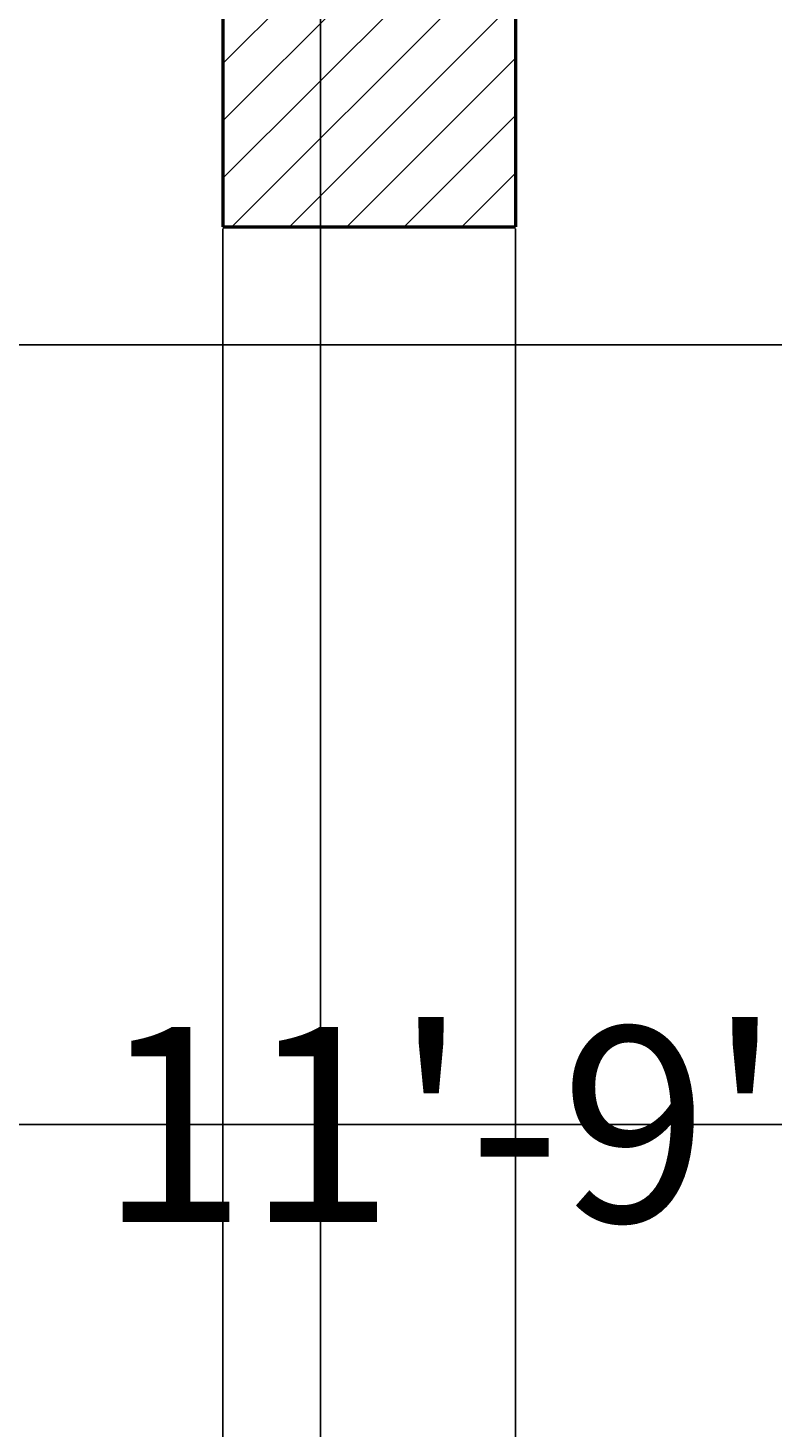
# Model space of a CAD drawing. Units: inches. Extents: x 0 to 281, y -535 to 46.
# Tile 8 of 22: x 150 to 173, y -168 to -125. Entities that reach past the tile are written whole.
import ezdxf

# ---------------------------------------------------------------- set-up
doc = ezdxf.new("R2010")
doc.units = ezdxf.units.IN
doc.header["$MEASUREMENT"] = 0
for name, color, linetype, lineweight in [('A-ANNO-DIMS', 2, 'Continuous', 18), ('A-COLS', 7, 'Continuous', 50), ('A-COLS-PATT', 152, 'Continuous', 13), ('A-WALL', 7, 'Continuous', 50)]:
    doc.layers.add(name, color=color, linetype=linetype, lineweight=lineweight)
doc.styles.get("Standard").update_dxf_attribs({"font": 'arial.ttf'})
doc.dimstyles.get("Standard").update_dxf_attribs({"dimtxt": 0.18, "dimasz": 0.18, "dimexe": 0.18, "dimexo": 0.0625, "dimgap": 0.09, "dimtad": 0, "dimtih": 1, "dimtoh": 1, "dimdec": 0, "dimzin": 0, "dimdsep": 46, "dimlunit": 3, "dimtxsty": 'Standard', "dimcen": 0.09, "dimadec": 0, "dimazin": 0, "dimtfac": 1, "dimtdec": 0, "dimtofl": 0, "dimtmove": 0, "dimatfit": 3, "dimfxl": 1, "dimtolj": 1, "dimtzin": 0, "dimarcsym": 0})

# ---------------------------------------------------------------- blocks, each defined once
blk = doc.blocks.new('*D5')
at = {"layer": 'A-ANNO-DIMS', "color": 0, "lineweight": -2, "transparency": 16777216}
for p, q in [((93.459, -158.989), (93.459, -158.871)), ((93.639, -159.051), (153.846, -159.051)), ((234.279, -159.051), (174.072, -159.051)), ((234.459, -158.989), (234.459, -158.871))]:
    blk.add_line(p, q, dxfattribs=at)
at = {"layer": 'A-ANNO-DIMS', "color": 0, "transparency": 16777216}
for points in [[(93.639, -159.021), (93.639, -159.081), (93.459, -159.051)], [(234.279, -159.021), (234.279, -159.081), (234.459, -159.051)]]:
    blk.add_solid(points, dxfattribs=at)
at = {"layer": 'Defpoints', "color": 0, "transparency": 16777216}
for p in [(93.459, -159.051), (234.459, -159.051), (234.459, -159.051)]:
    blk.add_point(p, dxfattribs=at)
at = {"layer": 'A-ANNO-DIMS', "color": 0, "transparency": 16777216, "insert": (163.959, -159.051), "char_height": 6, "attachment_point": 5}
blk.add_mtext('\\A1;11\'-9"', dxfattribs=at)
blk = doc.blocks.new('*D41')
at = {"layer": 'A-ANNO-DIMS', "color": 0, "lineweight": -2, "transparency": 16777216}
for p, q in [((120.459, -131.473), (120.459, -535.041)), ((156.459, -131.473), (156.459, -535.041)), ((120.639, -534.861), (138.13, -534.861)), ((156.279, -534.861), (138.788, -534.861))]:
    blk.add_line(p, q, dxfattribs=at)
at = {"layer": 'A-ANNO-DIMS', "color": 0, "transparency": 16777216}
for points in [[(120.639, -534.831), (120.639, -534.891), (120.459, -534.861)], [(156.279, -534.831), (156.279, -534.891), (156.459, -534.861)]]:
    blk.add_solid(points, dxfattribs=at)
at = {"layer": 'Defpoints', "color": 0, "transparency": 16777216}
for p in [(120.459, -131.411), (156.459, -131.411), (156.459, -534.861)]:
    blk.add_point(p, dxfattribs=at)
at = {"layer": 'A-ANNO-DIMS', "color": 0, "transparency": 16777216, "insert": (138.459, -534.861), "char_height": 0.18, "attachment_point": 5}
blk.add_mtext('\\A1;3\'-0"', dxfattribs=at)
blk = doc.blocks.new('*D42')
at = {"layer": 'A-ANNO-DIMS', "color": 0, "lineweight": -2, "transparency": 16777216}
for p, q in [((165.459, -131.473), (165.459, -535.041)), ((189.459, -131.473), (189.459, -535.041)), ((165.639, -534.861), (177.128, -534.861)), ((189.279, -534.861), (177.79, -534.861))]:
    blk.add_line(p, q, dxfattribs=at)
at = {"layer": 'A-ANNO-DIMS', "color": 0, "transparency": 16777216}
for points in [[(165.639, -534.831), (165.639, -534.891), (165.459, -534.861)], [(189.279, -534.831), (189.279, -534.891), (189.459, -534.861)]]:
    blk.add_solid(points, dxfattribs=at)
at = {"layer": 'Defpoints', "color": 0, "transparency": 16777216}
for p in [(165.459, -131.411), (189.459, -131.411), (189.459, -534.861)]:
    blk.add_point(p, dxfattribs=at)
at = {"layer": 'A-ANNO-DIMS', "color": 0, "transparency": 16777216, "insert": (177.459, -534.861), "char_height": 0.18, "attachment_point": 5}
blk.add_mtext('\\A1;2\'-0"', dxfattribs=at)
blk = doc.blocks.new('*D43')
at = {"layer": 'A-ANNO-DIMS', "color": 0, "lineweight": -2, "transparency": 16777216}
for p, q in [((93.521, -135.051), (271.089, -135.051)), ((270.909, -135.231), (270.909, -146.869)), ((270.909, -158.871), (270.909, -147.233)), ((93.521, -159.051), (271.089, -159.051))]:
    blk.add_line(p, q, dxfattribs=at)
at = {"layer": 'A-ANNO-DIMS', "color": 0, "transparency": 16777216}
for points in [[(270.879, -135.231), (270.939, -135.231), (270.909, -135.051)], [(270.879, -158.871), (270.939, -158.871), (270.909, -159.051)]]:
    blk.add_solid(points, dxfattribs=at)
at = {"layer": 'Defpoints', "color": 0, "transparency": 16777216}
for p in [(93.459, -135.051), (93.459, -159.051), (270.909, -159.051)]:
    blk.add_point(p, dxfattribs=at)
at = {"layer": 'A-ANNO-DIMS', "color": 0, "transparency": 16777216, "insert": (270.909, -147.051), "char_height": 0.18, "attachment_point": 5}
blk.add_mtext('\\A1;2\'-0"', dxfattribs=at)
blk = doc.blocks.new('*D46')
at = {"layer": 'A-ANNO-DIMS', "color": 0, "lineweight": -2, "transparency": 16777216}
for p, q in [((159.459, -263.348), (159.459, 46.219)), ((195.459, -263.348), (195.459, 46.219)), ((159.639, 46.039), (177.13, 46.039)), ((195.279, 46.039), (177.788, 46.039))]:
    blk.add_line(p, q, dxfattribs=at)
at = {"layer": 'A-ANNO-DIMS', "color": 0, "transparency": 16777216}
for points in [[(159.639, 46.069), (159.639, 46.009), (159.459, 46.039)], [(195.279, 46.069), (195.279, 46.009), (195.459, 46.039)]]:
    blk.add_solid(points, dxfattribs=at)
at = {"layer": 'Defpoints', "color": 0, "transparency": 16777216}
for p in [(195.459, 46.039), (159.459, -263.411), (195.459, -263.411)]:
    blk.add_point(p, dxfattribs=at)
at = {"layer": 'A-ANNO-DIMS', "color": 0, "transparency": 16777216, "insert": (177.459, 46.039), "char_height": 0.18, "attachment_point": 5}
blk.add_mtext('\\A1;3\'-0"', dxfattribs=at)
blk = doc.blocks.new('*D48')
at = {"layer": 'A-ANNO-DIMS', "color": 0, "lineweight": -2, "transparency": 16777216}
for p, q in [((159.459, -392.348), (159.459, 46.219)), ((195.459, -392.348), (195.459, 46.219)), ((159.639, 46.039), (177.13, 46.039)), ((195.279, 46.039), (177.788, 46.039))]:
    blk.add_line(p, q, dxfattribs=at)
at = {"layer": 'A-ANNO-DIMS', "color": 0, "transparency": 16777216}
for points in [[(159.639, 46.069), (159.639, 46.009), (159.459, 46.039)], [(195.279, 46.069), (195.279, 46.009), (195.459, 46.039)]]:
    blk.add_solid(points, dxfattribs=at)
at = {"layer": 'Defpoints', "color": 0, "transparency": 16777216}
for p in [(195.459, 46.039), (159.459, -392.411), (195.459, -392.411)]:
    blk.add_point(p, dxfattribs=at)
at = {"layer": 'A-ANNO-DIMS', "color": 0, "transparency": 16777216, "insert": (177.459, 46.039), "char_height": 0.18, "attachment_point": 5}
blk.add_mtext('\\A1;3\'-0"', dxfattribs=at)

msp = doc.modelspace()

# ---------------------------------------------------------------- hatches: boundary and pattern name
at = {"layer": 'A-COLS-PATT'}
h = msp.add_hatch(dxfattribs=at)
h.set_pattern_fill('ANSI31', color=256, scale=10)
h.paths.add_polyline_path([(165.459, -122.411), (156.459, -122.411), (156.459, -131.411), (165.459, -131.411)])
h.paths.add_polyline_path([(159.459, -263.411), (150.459, -263.411), (150.459, -272.411), (159.459, -272.411)])

# ---------------------------------------------------------------- linework, layer by layer
at = {"layer": 'A-COLS'}
msp.add_line((156.459, -131.411), (165.459, -131.411), dxfattribs=at)
at = {"layer": 'A-WALL'}
for p, q in [((156.459, 18.589), (156.459, -131.411)), ((165.459, 18.589), (165.459, -131.411))]:
    msp.add_line(p, q, dxfattribs=at)

# ---------------------------------------------------------------- dimensions: what is measured, and where the dimension line sits
at = {"layer": 'A-ANNO-DIMS'}
for base, p1, p2, override, picture, middle in [((195.459, 46.039), (159.459, -263.411), (195.459, -263.411), {"dimdec": 1, "dimlfac": 1, "dimrnd": 0, "dimzin": 1, "dimdsep": 46, "dimlunit": 4, "dimfrac": 2}, '*D46', (177.459, 46.039)), ((195.459, 46.039), (159.459, -392.411), (195.459, -392.411), {"dimdec": 1, "dimlfac": 1, "dimrnd": 0, "dimzin": 1, "dimdsep": 46, "dimlunit": 4, "dimfrac": 2}, '*D48', (177.459, 46.039)), ((156.459, -534.861), (120.459, -131.411), (156.459, -131.411), {"dimdec": 1, "dimlfac": 1, "dimrnd": 0, "dimzin": 1, "dimdsep": 46, "dimlunit": 4, "dimfrac": 2}, '*D41', (138.459, -534.861)), ((189.459, -534.861), (165.459, -131.411), (189.459, -131.411), {"dimdec": 1, "dimlfac": 1, "dimrnd": 0, "dimzin": 1, "dimdsep": 46, "dimlunit": 4, "dimfrac": 2}, '*D42', (177.459, -534.861)), ((234.459, -159.051), (93.459, -159.051), (234.459, -159.051), {"dimtxt": 6, "dimclrd": 0, "dimclre": 0, "dimclrt": 0}, '*D5', (163.959, -159.051))]:
    dim = msp.add_linear_dim(base=base, p1=p1, p2=p2, dimstyle='Standard', override=override, dxfattribs=at)
    dim.commit()
    dim.dimension.update_dxf_attribs({"geometry": picture, "text_midpoint": middle})
dim = msp.add_linear_dim(base=(270.909, -159.051), p1=(93.459, -135.051), p2=(93.459, -159.051), angle=90, dimstyle='Standard', override={"dimdec": 1, "dimlfac": 1, "dimrnd": 0, "dimzin": 1, "dimdsep": 46, "dimlunit": 4, "dimfrac": 2}, dxfattribs=at)
dim.commit()
dim.dimension.update_dxf_attribs({"geometry": '*D43', "text_midpoint": (270.909, -147.051)})

doc.saveas('drawing.dxf')
